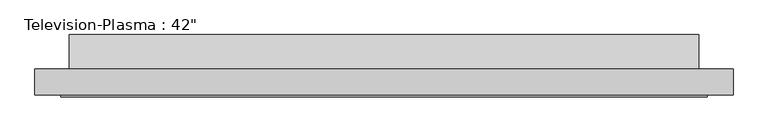
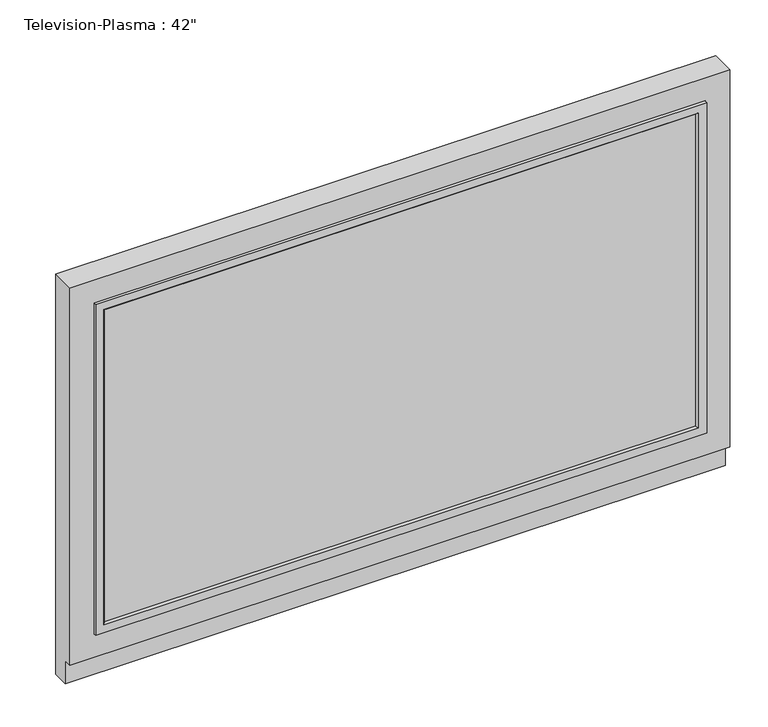
"""IFC4 building model written with IfcOpenShell, lengths in millimetres: furniture geometry."""

from ifc_helpers import new_model, si_unit, frame, origin, place, context, project, spatial, polyline, outline, extrude, faceted_brep, source, transform, mapped, element, save


def furniture_b6aab1a0(model_context):
    return source(origin(), model_context, "Body", "SolidModel", [
        extrude(outline(polyline([(520.7, -88.9), (-406.4, -88.9), (-406.4, -74.1720413), (520.7, -74.1720413), (520.7, -88.9)])), frame((0.0, 0.0, 88.9), z_axis=(0.0, 0.0, 1.0), x_axis=(1.0, 0.0, 0.0)), (0.0, 0.0, 1.0), 520.7),
        faceted_brep([(571.5, -50.8, 660.4), (-457.2, -50.8, 660.4), (-457.2, -88.9, 660.4), (571.5, -88.9, 660.4), (-457.2, -50.8, 0.0), (571.5, -50.8, 0.0), (571.5, -76.2, 0.0), (-457.2, -76.2, 0.0), (-406.4, -50.8, 609.6), (-406.4, -50.8, 38.1), (520.7, -50.8, 38.1), (520.7, -50.8, 609.6), (-457.2, -76.2, 38.1), (-457.2, -88.9, 38.1), (571.5, -88.9, 38.1), (-419.1, -88.9, 622.3), (533.4, -88.9, 622.3), (533.4, -88.9, 621.50625), (533.4, -88.9, 76.2), (-419.1, -88.9, 76.2), (-419.1, -88.9, 621.50625), (571.5, -76.2, 38.1), (533.4, -74.1720413, 622.3), (-419.1, -74.1720413, 622.3), (-419.1, -74.1720413, 621.50625), (533.4, -74.1720413, 621.50625), (520.7, -74.1720413, 88.9), (520.7, -74.1720413, 608.80625), (-406.4, -74.1720413, 608.80625), (-406.4, -74.1720413, 88.9), (-406.4, 0.0, 574.8688953), (-406.4, 0.0, 38.1), (520.7, 0.0, 574.8688953), (520.7, 0.0, 38.1), (517.525, -88.9, 92.075), (520.7, -92.075, 88.9), (520.7, -92.075, 608.80625), (517.525, -88.9, 605.63125), (520.7, -88.9, 88.9), (520.7, -88.9, 608.80625), (533.4, -92.075, 621.50625), (533.4, -92.075, 76.2), (-406.4, -92.075, 608.80625), (-403.225, -88.9, 605.63125), (-406.4, -88.9, 608.80625), (-419.1, -92.075, 621.50625), (-406.4, -92.075, 88.9), (-403.225, -88.9, 92.075), (-406.4, -88.9, 88.9), (-419.1, -92.075, 76.2)], [[[0, 1, 2, 3]], [[4, 5, 6, 7]], [[1, 0, 5, 4], [8, 9, 10, 11]], [[2, 1, 4, 7, 12, 13]], [[3, 2, 13, 14], [15, 16, 17, 18, 19, 20]], [[0, 3, 14, 21, 6, 5]], [[22, 23, 24, 25]], [[26, 27, 28, 29]], [[16, 22, 25, 17]], [[23, 15, 20, 24]], [[23, 22, 16, 15]], [[21, 12, 7, 6]], [[12, 21, 14, 13]], [[30, 31, 9, 8]], [[32, 11, 10, 33]], [[31, 30, 32, 33]], [[9, 31, 33, 10]], [[30, 8, 11, 32]], [[34, 35, 36, 37]], [[26, 38, 39, 27]], [[40, 41, 18, 17]], [[37, 36, 42, 43]], [[27, 39, 44, 28]], [[45, 40, 17, 25, 24, 20]], [[43, 42, 46, 47]], [[28, 44, 48, 29]], [[49, 45, 20, 19]], [[41, 40, 45, 49], [36, 35, 46, 42]], [[35, 34, 47, 46]], [[39, 38, 48, 44], [34, 37, 43, 47]], [[38, 26, 29, 48]], [[41, 49, 19, 18]]]),
    ])


if __name__ == "__main__":
    model = new_model("IFC4")
    model_context = context("Model", 3, world=origin())
    ifc_project = project(units=[si_unit("LENGTHUNIT", "METRE", prefix="MILLI")], contexts=[model_context])
    site = spatial("IfcSite", under=ifc_project)
    building = spatial("IfcBuilding", under=site)
    placement = place(None, origin())
    furniture_shape = furniture_b6aab1a0(model_context)
    element("IfcFurniture", 1, ObjectType="Television-Plasma : 42\"", at=placement, inside=building, context=model_context, shape_type="MappedRepresentation", body=[
        mapped(furniture_shape, transform((0.0, 0.0, 0.0), x_axis=(1.0, 0.0, 0.0), y_axis=(0.0, 1.0, 0.0), z_axis=(0.0, 0.0, 1.0))),
    ])
    save(model, "model.ifc")

# Revit data of these elements
# Type "Television-Plasma : 42\""
#   Assembly Code = "E2020200"
#   Depth = 0' - 3 1/2"
#   Height = 2' - 2"
#   Width = 3' - 4 1/2"
#   Cabinet Material = Plastic - Gray
#   Default Elevation = 0
# Element 1 (IfcFurniture, "Television-Plasma : 42\"")
#   Materials on its faces: "Plastic - Gray", "Glass"
# Materials
#   "Plastic - Gray": colour RGB 134 134 134, transparency 0
#   "Glass": class "Glass", colour RGB 0 128 192, transparency 0.75, Description = "Soda Lime Glass", Cost = 0
